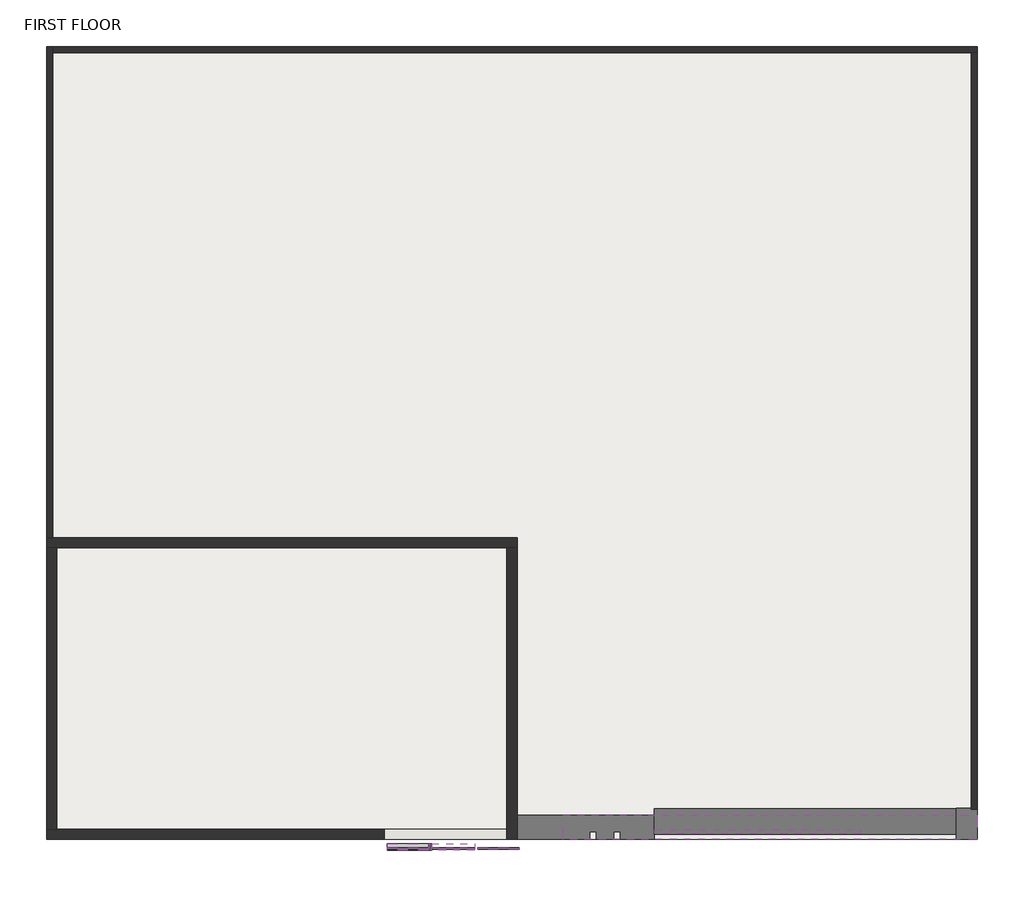
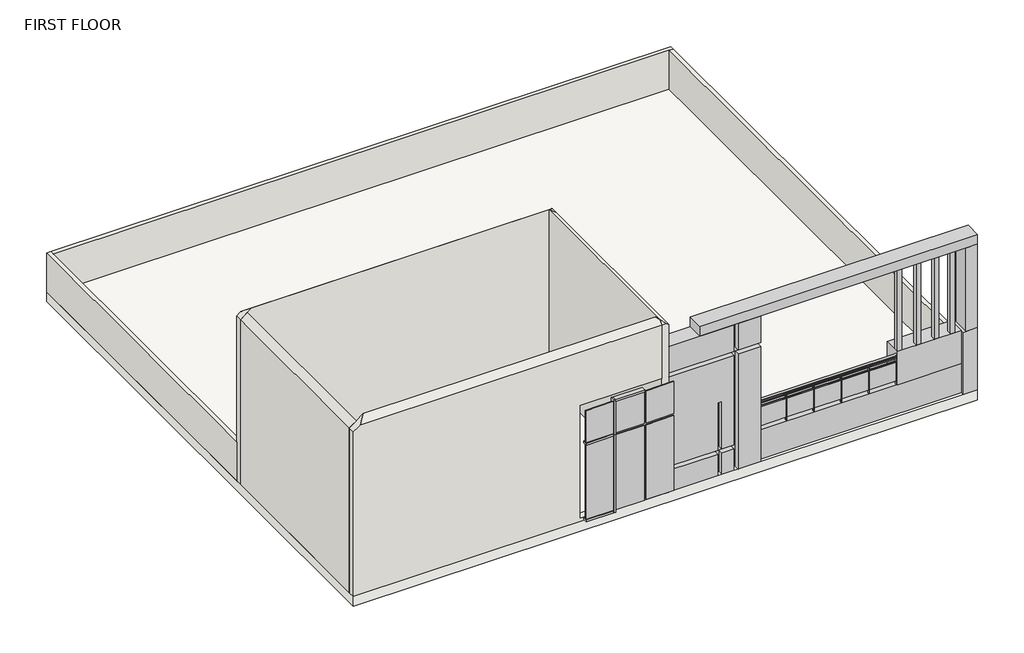
# One storey: 7 walls, 6 plates, 5 members, 2 proxies, 1 railing, 1 roof.
"""IFC4 building model written with IfcOpenShell, lengths in millimetres."""

from ifc_helpers import new_model, si_unit, point, frame, origin, place, context, project, spatial, polyline, ellipse_curve, trimmed, outline, extrude, faceted_brep, transform, mapped, element, save
from ifc_brep_helpers import plane_surface, extruded_surface, advanced_brep
from components import generic_models_2_generic_models_2_1caf7409, generic_models_9_generic_models_9_faf0bcb1, member_f0fea5a5, member_b90701c7, member_bef5179f, member_a085fe98, member_9b18e963, system_panel_glazed_ad069301, system_panel_glazed_46c6fbea, system_panel_glazed_ea0d7bad, system_panel_glazed_c42ef2fd

model = new_model("IFC4")

# Units and contexts
model_context = context("Model", 3, world=origin())
ifc_project = project(units=[si_unit("LENGTHUNIT", "METRE", prefix="MILLI")], contexts=[model_context])

# Site, building, storey
site = spatial("IfcSite", under=ifc_project)
building = spatial("IfcBuilding", under=site)
storey = spatial("IfcBuildingStorey", under=building, Name="FIRST FLOOR", Elevation=3048.0)

# Proxies
placement = place(None, origin())
generic_models_2_generic_models_2_shape = generic_models_2_generic_models_2_1caf7409(model_context)
element("IfcBuildingElementProxy", 1, Name="Generic Models 2 : Generic Models 2", ObjectType="Generic Models 2 : Generic Models 2", at=placement, inside=storey, context=model_context, shape_type="MappedRepresentation", body=[
    mapped(generic_models_2_generic_models_2_shape, transform((0.0, 0.0, 0.0), x_axis=(1.0, 0.0, 0.0), y_axis=(0.0, 1.0, 0.0), z_axis=(0.0, 0.0, 1.0))),
])
generic_models_9_generic_models_9_shape = generic_models_9_generic_models_9_faf0bcb1(model_context)
element("IfcBuildingElementProxy", 2, Name="Generic Models 9 : Generic Models 9", ObjectType="Generic Models 9 : Generic Models 9", at=placement, inside=storey, context=model_context, shape_type="MappedRepresentation", body=[
    mapped(generic_models_9_generic_models_9_shape, transform((0.0, 0.0, 0.0), x_axis=(1.0, 0.0, 0.0), y_axis=(0.0, 1.0, 0.0), z_axis=(0.0, 0.0, 1.0))),
])

# Members
member_shape = member_f0fea5a5(model_context)
element("IfcMember", 3, ObjectType="Rectangular Mullion : 2.5\" x 5\" rectangular", at=placement, inside=storey, context=model_context, shape_type="MappedRepresentation", body=[
    mapped(member_shape, transform((-1137.6455732, -4263.874389, 3450.2081328), x_axis=(-1.0, 0.0, 0.0), y_axis=(0.0, 1.0, 0.0), z_axis=(0.0, 0.0, -1.0))),
])
member_2_shape = member_b90701c7(model_context)
element("IfcMember", 4, ObjectType="Rectangular Mullion : 2.5\" x 5\" rectangular", at=placement, inside=storey, context=model_context, shape_type="MappedRepresentation", body=[
    mapped(member_2_shape, transform((-1137.6455732, -4263.874389, 5888.6081328), x_axis=(-1.0, 0.0, 0.0), y_axis=(0.0, 1.0, 0.0), z_axis=(0.0, 0.0, -1.0))),
])
member_3_shape = member_bef5179f(model_context)
element("IfcMember", 5, ObjectType="Rectangular Mullion : 2.5\" x 5\" rectangular", at=placement, inside=storey, context=model_context, shape_type="MappedRepresentation", body=[
    mapped(member_3_shape, transform((-1169.3955732, -4263.874389, 3450.2081328), x_axis=(0.0, 0.0, -1.0), y_axis=(0.0, 1.0, 0.0), z_axis=(1.0, 0.0, 0.0))),
])
member_4_shape = member_a085fe98(model_context)
element("IfcMember", 6, ObjectType="Rectangular Mullion : 2.5\" x 5\" rectangular", at=placement, inside=storey, context=model_context, shape_type="MappedRepresentation", body=[
    mapped(member_4_shape, transform((-1988.5455733, -4263.874389, 5888.6081328), x_axis=(0.0, 0.0, 1.0), y_axis=(0.0, 1.0, 0.0), z_axis=(-1.0, 0.0, 0.0))),
])
member_5_shape = member_9b18e963(model_context)
element("IfcMember", 7, ObjectType="Rectangular Mullion : 2.5\" x 5\" rectangular", at=placement, inside=storey, context=model_context, shape_type="MappedRepresentation", body=[
    mapped(member_5_shape, transform((-1105.8955732, -4263.874389, 6988.1851727), x_axis=(0.0, 0.0, 1.0), y_axis=(0.0, 1.0, 0.0), z_axis=(-1.0, 0.0, 0.0))),
])

# Plates
system_panel_glazed_shape = system_panel_glazed_ad069301(model_context)
element("IfcPlate", 8, ObjectType="System Panel : Glazed", at=placement, inside=storey, context=model_context, shape_type="MappedRepresentation", body=[
    mapped(system_panel_glazed_shape, transform((218.0794267, -4263.874389, 3513.7081328), x_axis=(-1.0, 0.0, 0.0), y_axis=(0.0, -1.0, 0.0), z_axis=(0.0, 0.0, 1.0))),
])
element("IfcPlate", 9, ObjectType="System Panel : Glazed", at=placement, inside=storey, context=model_context, shape_type="MappedRepresentation", body=[
    mapped(system_panel_glazed_shape, transform((-1578.9705732, -4263.874389, 3513.7081328), x_axis=(-1.0, 0.0, 0.0), y_axis=(0.0, -1.0, 0.0), z_axis=(0.0, 0.0, 1.0))),
])
system_panel_glazed_2_shape = system_panel_glazed_46c6fbea(model_context)
element("IfcPlate", 10, ObjectType="System Panel : Glazed", at=placement, inside=storey, context=model_context, shape_type="MappedRepresentation", body=[
    mapped(system_panel_glazed_2_shape, transform((218.0794267, -4263.874389, 5920.3581328), x_axis=(-1.0, 0.0, 0.0), y_axis=(0.0, -1.0, 0.0), z_axis=(0.0, 0.0, 1.0))),
])
element("IfcPlate", 11, ObjectType="System Panel : Glazed", at=placement, inside=storey, context=model_context, shape_type="MappedRepresentation", body=[
    mapped(system_panel_glazed_2_shape, transform((-1578.9705732, -4263.874389, 5920.3581328), x_axis=(-1.0, 0.0, 0.0), y_axis=(0.0, -1.0, 0.0), z_axis=(0.0, 0.0, 1.0))),
])
system_panel_glazed_3_shape = system_panel_glazed_ea0d7bad(model_context)
element("IfcPlate", 12, ObjectType="System Panel : Glazed", at=placement, inside=storey, context=model_context, shape_type="MappedRepresentation", body=[
    mapped(system_panel_glazed_3_shape, transform((-680.4455733, -4263.874389, 3513.7081328), x_axis=(-1.0, 0.0, 0.0), y_axis=(0.0, -1.0, 0.0), z_axis=(0.0, 0.0, 1.0))),
])
system_panel_glazed_4_shape = system_panel_glazed_c42ef2fd(model_context)
element("IfcPlate", 13, ObjectType="System Panel : Glazed", at=placement, inside=storey, context=model_context, shape_type="MappedRepresentation", body=[
    mapped(system_panel_glazed_4_shape, transform((-680.4455733, -4263.874389, 5920.3581328), x_axis=(-1.0, 0.0, 0.0), y_axis=(0.0, -1.0, 0.0), z_axis=(0.0, 0.0, 1.0))),
])

# Railing
element("IfcRailing", 14, ObjectType="Glass Panel - Bottom Fill", at=placement, inside=storey, context=model_context, shape_type="SolidModel", body=[
    advanced_brep(
    [(7416.0108478, -3997.174389, 5181.6), (7416.0108478, -3920.974389, 5181.6), (3326.6108478, -3997.174389, 5181.6), (3326.6108478, -3920.974389, 5181.6)],
    [
        (0, 1, ellipse_curve(frame((7416.0108478, -3959.074389, 5181.6), z_axis=(1.0, 0.0, 0.0), x_axis=(0.0, 1.0, 0.0)), 38.1, 28.575)),
        (1, 0, ellipse_curve(frame((7416.0108478, -3959.074389, 5181.6), z_axis=(1.0, 0.0, 0.0), x_axis=(0.0, 1.0, 0.0)), 38.1, 28.575)),
        (2, 3, ellipse_curve(frame((3326.6108478, -3959.074389, 5181.6), z_axis=(-1.0, 0.0, 0.0), x_axis=(0.0, 1.0, 0.0)), 38.1, 28.575)),
        (3, 2, ellipse_curve(frame((3326.6108478, -3959.074389, 5181.6), z_axis=(-1.0, 0.0, 0.0), x_axis=(0.0, 1.0, 0.0)), 38.1, 28.575)),
        (0, 2),
        (3, 1),
    ],
    [
        plane_surface(frame((7416.0108478, -3959.074389, 5181.6), z_axis=(1.0, 0.0, 0.0), x_axis=(0.0, -1.0, 0.0))),
        plane_surface(frame((3326.6108478, -3959.074389, 5181.6), z_axis=(-1.0, 0.0, 0.0), x_axis=(0.0, -1.0, 0.0))),
        extruded_surface(trimmed(ellipse_curve(frame((3326.6108478, -3959.074389, 5181.6), z_axis=(1.0, 0.0, 0.0), x_axis=(0.0, 1.0, 0.0)), 38.1, 28.575), [point((3326.6108478, -3997.174389, 5181.6))], [point((3326.6108478, -3920.974389, 5181.6))], True, "CARTESIAN"), (4089.4, 0.0, 0.0), 4089.4),
        extruded_surface(trimmed(ellipse_curve(frame((3326.6108478, -3959.074389, 5181.6), z_axis=(1.0, 0.0, 0.0), x_axis=(0.0, 1.0, 0.0)), 38.1, 28.575), [point((3326.6108478, -3920.974389, 5181.6))], [point((3326.6108478, -3997.174389, 5181.6))], True, "CARTESIAN"), (4089.4, 0.0, 0.0), 4089.4),
    ],
    [
        (0, [[1, 2]]),
        (1, [[3, 4]]),
        (2, [[-1, 5, -4, 6]]),
        (3, [[-2, -6, -3, -5]]),
    ],
),
    extrude(outline(polyline([(7416.0108478, -3946.374389), (7416.0108478, -3971.774389), (3326.6108478, -3971.774389), (3326.6108478, -3946.374389), (7416.0108478, -3946.374389)])), frame((0.0, 0.0, 5067.3), z_axis=(0.0, 0.0, 1.0), x_axis=(1.0, 0.0, 0.0)), (0.0, 0.0, 1.0), 25.4),
    extrude(outline(polyline([(7416.0108478, -3946.374389), (7416.0108478, -3971.774389), (3326.6108478, -3971.774389), (3326.6108478, -3946.374389), (7416.0108478, -3946.374389)])), frame((0.0, 0.0, 4965.7), z_axis=(0.0, 0.0, 1.0), x_axis=(1.0, 0.0, 0.0)), (0.0, 0.0, 1.0), 25.4),
    extrude(outline(polyline([(3345.6608478, -3933.674389), (3345.6608478, -3984.474389), (3332.9608478, -3984.474389), (3332.9608478, -3933.674389), (3345.6608478, -3933.674389)])), frame((0.0, 0.0, 4267.2), z_axis=(0.0, 0.0, 1.0), x_axis=(1.0, 0.0, 0.0)), (0.0, 0.0, 1.0), 885.825),
    extrude(outline(polyline([(4152.1108478, -3965.609546), (3339.3108478, -3965.609546), (3339.3108478, -3959.259546), (4152.1108478, -3959.259546), (4152.1108478, -3965.609546)])), frame((0.0, 0.0, 4368.8), z_axis=(0.0, 0.0, 1.0), x_axis=(1.0, 0.0, 0.0)), (0.0, 0.0, 1.0), 596.9),
    extrude(outline(polyline([(4158.4608478, -3933.674389), (4158.4608478, -3984.474389), (4145.7608478, -3984.474389), (4145.7608478, -3933.674389), (4158.4608478, -3933.674389)])), frame((0.0, 0.0, 4267.2), z_axis=(0.0, 0.0, 1.0), x_axis=(1.0, 0.0, 0.0)), (0.0, 0.0, 1.0), 885.825),
    extrude(outline(polyline([(4964.9108478, -3965.609546), (4152.1108478, -3965.609546), (4152.1108478, -3959.259546), (4964.9108478, -3959.259546), (4964.9108478, -3965.609546)])), frame((0.0, 0.0, 4368.8), z_axis=(0.0, 0.0, 1.0), x_axis=(1.0, 0.0, 0.0)), (0.0, 0.0, 1.0), 596.9),
    extrude(outline(polyline([(4971.2608478, -3933.674389), (4971.2608478, -3984.474389), (4958.5608478, -3984.474389), (4958.5608478, -3933.674389), (4971.2608478, -3933.674389)])), frame((0.0, 0.0, 4267.2), z_axis=(0.0, 0.0, 1.0), x_axis=(1.0, 0.0, 0.0)), (0.0, 0.0, 1.0), 885.825),
    extrude(outline(polyline([(5777.7108478, -3965.609546), (4964.9108478, -3965.609546), (4964.9108478, -3959.259546), (5777.7108478, -3959.259546), (5777.7108478, -3965.609546)])), frame((0.0, 0.0, 4368.8), z_axis=(0.0, 0.0, 1.0), x_axis=(1.0, 0.0, 0.0)), (0.0, 0.0, 1.0), 596.9),
    extrude(outline(polyline([(5784.0608478, -3933.674389), (5784.0608478, -3984.474389), (5771.3608478, -3984.474389), (5771.3608478, -3933.674389), (5784.0608478, -3933.674389)])), frame((0.0, 0.0, 4267.2), z_axis=(0.0, 0.0, 1.0), x_axis=(1.0, 0.0, 0.0)), (0.0, 0.0, 1.0), 885.825),
    extrude(outline(polyline([(6590.5108478, -3965.609546), (5777.7108478, -3965.609546), (5777.7108478, -3959.259546), (6590.5108478, -3959.259546), (6590.5108478, -3965.609546)])), frame((0.0, 0.0, 4368.8), z_axis=(0.0, 0.0, 1.0), x_axis=(1.0, 0.0, 0.0)), (0.0, 0.0, 1.0), 596.9),
    extrude(outline(polyline([(6596.8608478, -3933.674389), (6596.8608478, -3984.474389), (6584.1608478, -3984.474389), (6584.1608478, -3933.674389), (6596.8608478, -3933.674389)])), frame((0.0, 0.0, 4267.2), z_axis=(0.0, 0.0, 1.0), x_axis=(1.0, 0.0, 0.0)), (0.0, 0.0, 1.0), 885.825),
    extrude(outline(polyline([(7403.3108478, -3965.609546), (6590.5108478, -3965.609546), (6590.5108478, -3959.259546), (7403.3108478, -3959.259546), (7403.3108478, -3965.609546)])), frame((0.0, 0.0, 4368.8), z_axis=(0.0, 0.0, 1.0), x_axis=(1.0, 0.0, 0.0)), (0.0, 0.0, 1.0), 596.9),
    extrude(outline(polyline([(7409.6608478, -3933.674389), (7409.6608478, -3984.474389), (7396.9608478, -3984.474389), (7396.9608478, -3933.674389), (7409.6608478, -3933.674389)])), frame((0.0, 0.0, 4267.2), z_axis=(0.0, 0.0, 1.0), x_axis=(1.0, 0.0, 0.0)), (0.0, 0.0, 1.0), 885.825),
    extrude(outline(polyline([(3339.3108478, -3949.549389), (3339.3108478, -3968.599389), (3320.2608478, -3968.599389), (3320.2608478, -3949.549389), (3339.3108478, -3949.549389)])), frame((0.0, 0.0, 4267.2), z_axis=(0.0, 0.0, 1.0), x_axis=(1.0, 0.0, 0.0)), (0.0, 0.0, 1.0), 885.825),
    extrude(outline(polyline([(7422.3608478, -3949.549389), (7422.3608478, -3968.599389), (7403.3108478, -3968.599389), (7403.3108478, -3949.549389), (7422.3608478, -3949.549389)])), frame((0.0, 0.0, 4267.2), z_axis=(0.0, 0.0, 1.0), x_axis=(1.0, 0.0, 0.0)), (0.0, 0.0, 1.0), 885.825),
])

# Roof
element("IfcRoof", 15, ObjectType="Generic - 12\"", at=placement, inside=storey, context=model_context, shape_type="SweptSolid", body=[
    extrude(outline(polyline([(-8757.645593, 11636.525611), (9733.554407, 11636.525611), (9733.554407, -4111.474389), (-8757.645593, -4111.474389), (-8757.645593, 11636.525611)])), frame((0.0, 0.0, 3048.0), z_axis=(0.0, 0.0, 1.0), x_axis=(1.0, 0.0, 0.0)), (0.0, 0.0, 1.0), 304.8),
])

# Walls
element("IfcWall", 16, ObjectType="Generic - 5\"", at=placement, inside=storey, context=model_context, shape_type="Brep", body=[
    faceted_brep([(-8630.645593, 1882.925611, 3352.8), (-8630.645593, 11509.525611, 3352.8), (-8630.645593, 11636.525611, 3352.8), (-8630.645593, 11636.525611, 4572.0), (-8630.645593, 11509.525611, 4572.0), (-8630.645593, 1882.925611, 4572.0), (-8757.645593, 1882.925611, 3352.8), (-8757.645593, 1882.925611, 4572.0), (-8757.645593, 11636.525611, 4572.0), (-8757.645593, 11636.525611, 3352.8)], [[[0, 1, 2, 3, 4, 5]], [[6, 7, 8, 9]], [[2, 1, 0, 6, 9]], [[5, 4, 3, 8, 7]], [[0, 5, 7, 6]], [[3, 2, 9, 8]]]),
])
element("IfcWall", 17, ObjectType="Generic - 5\"", at=placement, inside=storey, context=model_context, shape_type="Brep", body=[
    faceted_brep([(-8630.645593, 11509.525611, 3352.8), (9606.554407, 11509.525611, 3352.8), (9733.554407, 11509.525611, 3352.8), (9733.554407, 11509.525611, 4572.0), (9606.554407, 11509.525611, 4572.0), (-8630.645593, 11509.525611, 4572.0), (-8630.645593, 11636.525611, 3352.8), (-8630.645593, 11636.525611, 4572.0), (9733.554407, 11636.525611, 4572.0), (9733.554407, 11636.525611, 3352.8)], [[[0, 1, 2, 3, 4, 5]], [[6, 7, 8, 9]], [[2, 1, 0, 6, 9]], [[5, 4, 3, 8, 7]], [[0, 5, 7, 6]], [[3, 2, 9, 8]]]),
])
element("IfcWall", 18, ObjectType="Generic - 5\"", at=placement, inside=storey, context=model_context, shape_type="SweptSolid", body=[
    extrude(outline(polyline([(9606.554407, -3514.574389), (9606.554407, 11509.525611), (9733.554407, 11509.525611), (9733.554407, -3514.574389), (9606.554407, -3514.574389)])), frame((0.0, 0.0, 3352.8), z_axis=(0.0, 0.0, 1.0), x_axis=(1.0, 0.0, 0.0)), (0.0, 0.0, 1.0), 1219.2),
])
element("IfcWall", 19, ObjectType="Generic - 8\"", at=placement, inside=storey, context=model_context, shape_type="Brep", body=[
    faceted_brep([(-8757.645593, 1679.725611, 8515.35), (-8757.645593, 1679.725611, 3352.8), (-8554.445593, 1679.725611, 3352.8), (386.354407, 1679.725611, 3352.8), (589.554407, 1679.725611, 3352.8), (589.554407, 1679.725611, 8610.6), (386.354407, 1679.725611, 8763.0), (-8427.445593, 1679.725611, 8763.0), (-8554.445593, 1679.725611, 8667.75), (-8757.645593, 1882.925611, 3352.8), (-8757.645593, 1882.925611, 4572.0), (-8757.645593, 1882.925611, 8515.35), (-8630.645593, 1882.925611, 8610.6), (589.554407, 1882.925611, 8610.6), (589.554407, 1882.925611, 3352.8), (-8630.645593, 1882.925611, 3352.8)], [[[0, 1, 2, 3, 4, 5, 6, 7, 8]], [[9, 10, 11, 12, 13, 14, 15]], [[4, 3, 2, 1, 9, 15, 14]], [[5, 4, 14, 13]], [[0, 11, 10, 9, 1]], [[0, 8, 7, 12, 11]], [[7, 6, 13, 12]], [[6, 5, 13]]]),
])
element("IfcWall", 20, ObjectType="Generic - 8\"", at=placement, inside=storey, context=model_context, shape_type="Brep", body=[
    faceted_brep([(386.354407, 1679.725611, 3352.8), (386.354407, -3908.274389, 3352.8), (386.354407, -4111.474389, 3352.8), (386.354407, -4111.474389, 8667.75), (386.354407, -3984.474389, 8763.0), (386.354407, -3908.274389, 8763.0), (386.354407, 1679.725611, 8763.0), (589.554407, 1679.725611, 3352.8), (589.554407, 1679.725611, 8610.6), (589.554407, -4111.474389, 8610.6), (589.554407, -4111.474389, 3352.8), (513.354407, -4111.474389, 8667.75)], [[[0, 1, 2, 3, 4, 5, 6]], [[7, 8, 9, 10]], [[2, 1, 0, 7, 10]], [[0, 6, 8, 7]], [[3, 2, 10, 9, 11]], [[6, 5, 4, 11, 9, 8]], [[4, 3, 11]]]),
])
element("IfcWall", 21, ObjectType="Generic - 8\"", at=placement, inside=storey, context=model_context, shape_type="Brep", body=[
    faceted_brep([(386.354407, -3908.274389, 3352.8), (-8554.445593, -3908.274389, 3352.8), (-8757.645593, -3908.274389, 3352.8), (-8757.645593, -3908.274389, 8515.35), (-8554.445593, -3908.274389, 8667.75), (-8351.245593, -3908.274389, 8820.15), (310.154407, -3908.274389, 8820.15), (386.354407, -3908.274389, 8763.0), (386.354407, -3908.274389, 6988.1851727), (-2052.0455733, -3908.274389, 6988.1851727), (-2052.0455733, -3908.274389, 3450.2081328), (386.354407, -3908.274389, 3450.2081328), (-8757.645593, -4111.474389, 3352.8), (386.354407, -4111.474389, 3352.8), (386.354407, -4111.474389, 3450.2081328), (-2052.0455733, -4111.474389, 3450.2081328), (-2052.0455733, -4111.474389, 6988.1851727), (386.354407, -4111.474389, 6988.1851727), (386.354407, -4111.474389, 8667.75), (-8554.445593, -4111.474389, 8667.75), (-8757.645593, -4111.474389, 8515.35), (386.354407, -3984.474389, 8763.0)], [[[0, 1, 2, 3, 4, 5, 6, 7, 8, 9, 10, 11]], [[12, 13, 14, 15, 16, 17, 18, 19, 20]], [[2, 1, 0, 13, 12]], [[13, 0, 11, 14]], [[21, 18, 17, 8, 7]], [[3, 2, 12, 20]], [[16, 9, 8, 17]], [[9, 16, 15, 10]], [[10, 15, 14, 11]], [[7, 6, 21]], [[6, 5, 19, 18, 21]], [[3, 20, 19, 5, 4]]]),
])
element("IfcWall", 22, ObjectType="Generic - 8\"", at=placement, inside=storey, context=model_context, shape_type="SweptSolid", body=[
    extrude(outline(polyline([(3352.8, -8554.445593), (8667.75, -8554.445593), (8515.35, -8757.645593), (3352.8, -8757.645593), (3352.8, -8554.445593)])), frame((0.0, -3908.274389, 0.0), z_axis=(0.0, 1.0, 0.0), x_axis=(0.0, 0.0, 1.0)), (0.0, 0.0, 1.0), 5588.0),
])

save(model, "model.ifc")

# Revit data of these elements
# Type "Rectangular Mullion : 2.5\" x 5\" rectangular"
#   built-in parameter 1007304 = 0.416667 (stored number, unit not read)
#   built-in parameter 1007301 = 0.104167 (stored number, unit not read)
#   built-in parameter 1007300 = 0.104167 (stored number, unit not read)
# Type "System Panel : Glazed"
#   Construction Type Id = "GSP4R"
#   Analytic Construction = "1/8 in Pilkington single glazing"
#   Visual Light Transmittance = 0.9
#   Solar Heat Gain Coefficient = 0.86
#   Heat Transfer Coefficient (U) = 1.18115 BTU/(h·ft²·°F)
#   Define Thermal Properties by = 1
# Type "Glass Panel - Bottom Fill"
#   Assembly Code = "C2010400"
#   built-in parameter 1008612 = 0.0416667 (stored number, unit not read)
#   built-in parameter 1008611 = 0.0416667 (stored number, unit not read)
#   built-in parameter 1008609 = 0.333333 (stored number, unit not read)
#   built-in parameter 1008604 = 0.166667 (stored number, unit not read)
#   built-in parameter 1008603 = 0.166667 (stored number, unit not read)
#   Railing Height = 3' - 0"
#   built-in parameter 1008630 = 2
#   built-in parameter 1008610 = 2
#   built-in parameter 1008618 = Baluster - Square : 3/4"
# Type "Generic - 12\""
#   Assembly Code = "B1020"
#   Layers, outside or top first: 1' - 0" "ROOFING MATERIAL" (function 1)
# Type "Generic - 5\""
#   Assembly Code = "B2010"
#   Layers, outside or top first: 0' - 5" no material (function 1)
# Type "Generic - 8\""
#   Assembly Code = "B2010"
#   Layers, outside or top first: 0' - 8" no material (function 1)
# Element 1 (IfcBuildingElementProxy, "Generic Models 2 : Generic Models 2")
#   Phase Created = New Construction
#   Materials on its faces: "Asphalt Shingle", "OLIVE GREY", "LIGHT GREY WHITE", "Wood Planks"
# Element 2 (IfcBuildingElementProxy, "Generic Models 9 : Generic Models 9")
#   Phase Created = New Construction
#   Materials on its faces: "TOP HORZ"
# Elements 3, 4, 5, 6, 7 (IfcMember, "Rectangular Mullion : 2.5\" x 5\" rectangular")
#   Phase Created = New Construction
#   Materials on its faces: "Aluminum"
# Elements 8, 9, 10, 11, 12, 13 (IfcPlate, "System Panel : Glazed")
#   Phase Created = New Construction
#   Materials on its faces: "Glass"
# Element 14 (IfcRailing, "Glass Panel - Bottom Fill")
#   built-in parameter 1008621 = 4 (stored number, unit not read)
#   Phase Created = New Construction
#   Materials on its faces: "Glass", "Iron, Ductile"
# Element 15 (IfcRoof, "Generic - 12\"")
#   built-in parameter 1001705 = 11 (stored number, unit not read)
#   built-in parameter 1001710 = 33615
#   Phase Created = New Construction
#   Materials on its faces: "Laminate, Ivory, Matte", "ROOFING MATERIAL"
# Elements 16, 17, 18 (IfcWall, "Generic - 5\"")
#   built-in parameter 1001111 = 1' - 0"
#   Top Offset = 0' - 0"
#   Base Offset = 1' - 0"
#   Unconnected Height = 4' - 0"
#   wall height = 4' - 0"
#   Phase Created = New Construction
#   Base Constraint = FIRST FLOOR
#   Materials on its faces: "Gypsum Wall Board", "Default Wall"
# Elements 19, 20, 21, 22 (IfcWall, "Generic - 8\"")
#   built-in parameter 1001111 = 1' - 0"
#   Top Offset = 0' - 0"
#   Base Offset = 1' - 0"
#   Unconnected Height = 15' - 0"
#   wall height = 15' - 0"
#   Phase Created = New Construction
#   Base Constraint = FIRST FLOOR
#   Materials on its faces: "Default Wall", "WHITE COLOUR FOR WALLS"
# Materials
#   "ROOFING MATERIAL": class "Generic", colour RGB 120 120 120, transparency 0, Cost = 0
#   "Asphalt Shingle": class "Generic", colour RGB 155 155 155, transparency 0, Description = "Asphalt roofing shingle", Cost = 0
#   "OLIVE GREY": class "Generic", colour RGB 120 120 120, transparency 0, Cost = 0
#   "LIGHT GREY WHITE": class "Generic", colour RGB 120 120 120, transparency 0, Cost = 0
#   "Wood Planks": class "Wood", colour RGB 193 160 115, transparency 0, Description = "Physical material.", Cost = 0
#   "TOP HORZ": class "Generic", colour RGB 120 120 120, transparency 0, Cost = 0
#   "Aluminum": class "Metal", colour RGB 247 247 247, transparency 0, Description = "Aluminum 6061", Cost = 0
#   "Glass": class "Glass", colour RGB 0 128 192, transparency 0.75, Description = "Soda Lime Glass", Cost = 0
#   "Iron, Ductile": class "Metal", colour RGB 0 0 0, transparency 0, Description = "Ductile cast iron", Cost = 0
#   "Laminate, Ivory, Matte": class "Plastic", colour RGB 247 247 239, transparency 0, Description = "Plastic Laminate - Ivory, Matte", Cost = 0
#   "Gypsum Wall Board": class "Generic", colour RGB 127 127 127, transparency 0, Description = "Gypsum Wall Board", Cost = 0
#   "Default Wall": colour RGB 128 128 128, transparency 0, Cost = 0
#   "WHITE COLOUR FOR WALLS": class "Generic", colour RGB 120 120 120, transparency 0, Cost = 0
